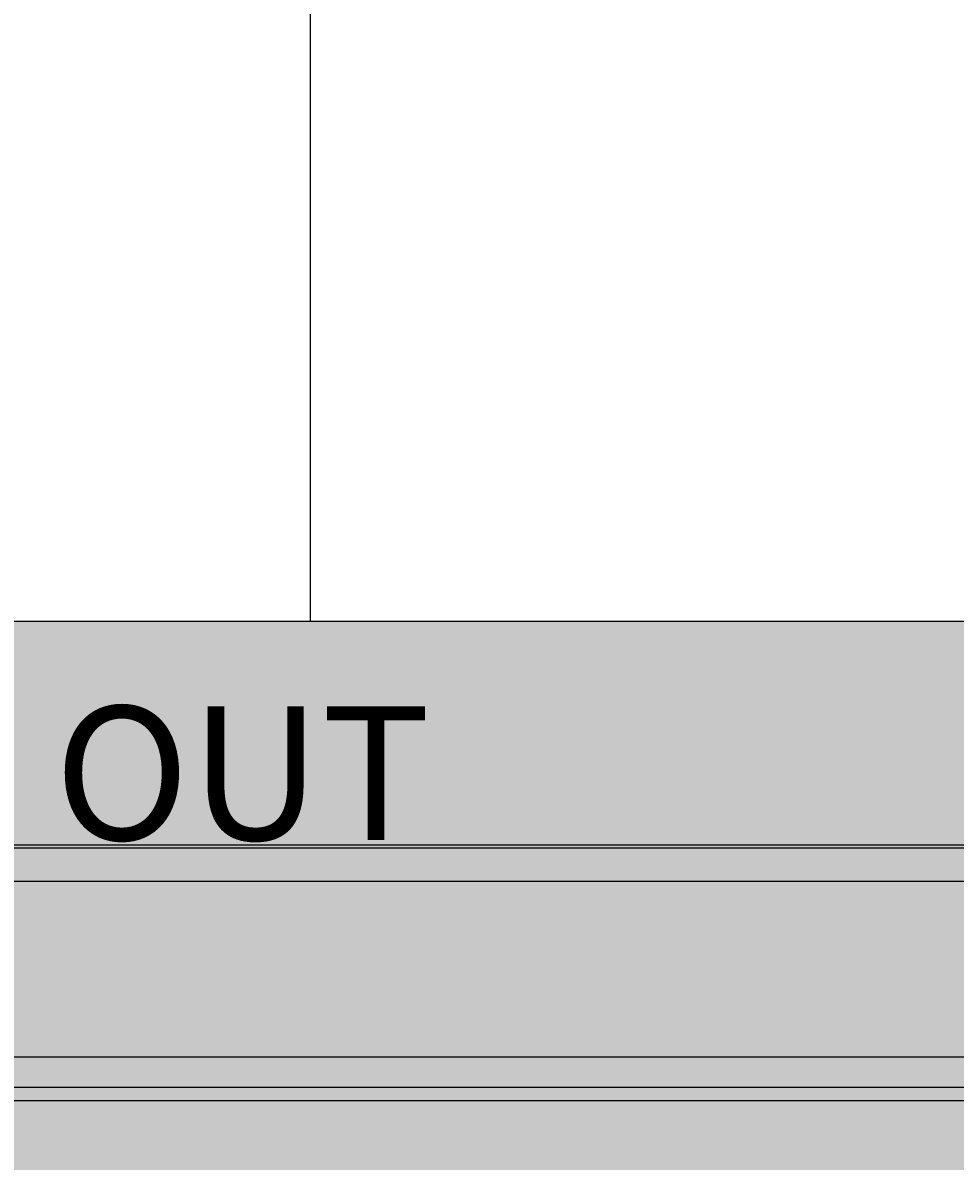
# Model space of a CAD drawing. Units: inches. Extents: x 35362 to 73946, y 43607 to 67532.
# Tile 64 of 134: x 46225 to 47763, y 48798 to 50677. Entities that reach past the tile are written whole.
import ezdxf

# ---------------------------------------------------------------- set-up
doc = ezdxf.new("R2010")
doc.units = ezdxf.units.IN
doc.header["$MEASUREMENT"] = 0
for name, color, linetype, lineweight in [('A-ANNO-DIMS', 2, 'Continuous', 18), ('E-ANNO-TEXT', 5, 'Continuous', 18), ('E-SYMB', 1, 'Continuous', 25), ('E-SYMB-PATT', 1, 'Continuous', 13), ('E-WIRE', 3, 'Continuous', 25)]:
    doc.layers.add(name, color=color, linetype=linetype, lineweight=lineweight)
doc.styles.get("Standard").update_dxf_attribs({"font": 'arial.ttf'})
doc.dimstyles.get("Standard").update_dxf_attribs({"dimtxt": 0.18, "dimasz": 0.18, "dimexe": 0.18, "dimexo": 0.0625, "dimgap": 0.09, "dimtad": 0, "dimtih": 1, "dimtoh": 1, "dimdec": 4, "dimzin": 0, "dimdsep": 46, "dimtxsty": 'Standard', "dimcen": 0.09, "dimadec": 0, "dimazin": 0, "dimtfac": 1, "dimtdec": 4, "dimtofl": 0, "dimtmove": 0, "dimatfit": 3, "dimfxl": 1, "dimtolj": 1, "dimtzin": 0, "dimarcsym": 0})

# ---------------------------------------------------------------- blocks, each defined once
blk = doc.blocks.new('*D40')
at = {"layer": 'A-ANNO-DIMS', "color": 0, "lineweight": -2, "transparency": 16777216}
for p, q in [((56873.5, 53351.5), (35361.8, 53351.5)), ((35361.9, 53351.3), (35361.9, 51333.3)), ((35361.9, 49314.8), (35361.9, 51332.9)), ((51806.5, 49314.7), (35361.8, 49314.7))]:
    blk.add_line(p, q, dxfattribs=at)
at = {"layer": 'A-ANNO-DIMS', "color": 0, "transparency": 16777216}
for points in [[(35361.9, 53351.3), (35362, 53351.3), (35361.9, 53351.5)], [(35361.9, 49314.8), (35362, 49314.8), (35361.9, 49314.7)]]:
    blk.add_solid(points, dxfattribs=at)
at = {"layer": 'Defpoints', "color": 0, "transparency": 16777216}
for p in [(35361.9, 53351.5), (56873.6, 53351.5), (51806.5, 49314.7)]:
    blk.add_point(p, dxfattribs=at)
at = {"layer": 'A-ANNO-DIMS', "color": 0, "transparency": 16777216, "insert": (35361.9, 51333.1), "char_height": 0.18, "attachment_point": 5}
blk.add_mtext('\\A1;4036.9', dxfattribs=at)
blk = doc.blocks.new('*D67')
at = {"layer": 'A-ANNO-DIMS', "color": 0, "lineweight": -2, "transparency": 16777216}
for p, q in [((56873.5, 53351.5), (35361.8, 53351.5)), ((35361.9, 53351.3), (35361.9, 49400.9)), ((35361.9, 45450.1), (35361.9, 49400.5)), ((53793.6, 45449.9), (35361.8, 45449.9))]:
    blk.add_line(p, q, dxfattribs=at)
at = {"layer": 'A-ANNO-DIMS', "color": 0, "transparency": 16777216}
for points in [[(35361.9, 53351.3), (35362, 53351.3), (35361.9, 53351.5)], [(35361.9, 45450.1), (35362, 45450.1), (35361.9, 45449.9)]]:
    blk.add_solid(points, dxfattribs=at)
at = {"layer": 'Defpoints', "color": 0, "transparency": 16777216}
for p in [(35361.9, 53351.5), (56873.6, 53351.5), (53793.6, 45449.9)]:
    blk.add_point(p, dxfattribs=at)
at = {"layer": 'A-ANNO-DIMS', "color": 0, "transparency": 16777216, "insert": (35361.9, 49400.7), "char_height": 0.18, "attachment_point": 5}
blk.add_mtext('\\A1;7901.6', dxfattribs=at)
blk = doc.blocks.new('*D84')
at = {"layer": 'A-ANNO-DIMS', "color": 0, "lineweight": -2, "transparency": 16777216}
for p, q in [((55540.2, 49259.9), (35361.8, 49259.9)), ((35361.9, 49259.8), (35361.9, 49115.1)), ((35361.9, 48970.2), (35361.9, 49114.8)), ((55540.2, 48970), (35361.8, 48970))]:
    blk.add_line(p, q, dxfattribs=at)
at = {"layer": 'A-ANNO-DIMS', "color": 0, "transparency": 16777216}
for points in [[(35361.9, 49259.8), (35362, 49259.8), (35361.9, 49259.9)], [(35361.9, 48970.2), (35362, 48970.2), (35361.9, 48970)]]:
    blk.add_solid(points, dxfattribs=at)
at = {"layer": 'Defpoints', "color": 0, "transparency": 16777216}
for p in [(35361.9, 49259.9), (55540.3, 49259.9), (55540.3, 48970)]:
    blk.add_point(p, dxfattribs=at)
at = {"layer": 'A-ANNO-DIMS', "color": 0, "transparency": 16777216, "insert": (35361.9, 49115), "char_height": 0.18, "attachment_point": 5}
blk.add_mtext('\\A1;289.96', dxfattribs=at)
blk = doc.blocks.new('*D86')
at = {"layer": 'A-ANNO-DIMS', "color": 0, "lineweight": -2, "transparency": 16777216}
for p, q in [((51285.5, 49320.1), (35361.8, 49320.1)), ((35361.9, 49319.9), (35361.9, 49120.3)), ((35361.9, 48920.3), (35361.9, 49119.9)), ((51285.5, 48920.1), (35361.8, 48920.1))]:
    blk.add_line(p, q, dxfattribs=at)
at = {"layer": 'A-ANNO-DIMS', "color": 0, "transparency": 16777216}
for points in [[(35361.9, 49319.9), (35362, 49319.9), (35361.9, 49320.1)], [(35361.9, 48920.3), (35362, 48920.3), (35361.9, 48920.1)]]:
    blk.add_solid(points, dxfattribs=at)
at = {"layer": 'Defpoints', "color": 0, "transparency": 16777216}
for p in [(35361.9, 49320.1), (51285.6, 49320.1), (51285.6, 48920.1)]:
    blk.add_point(p, dxfattribs=at)
at = {"layer": 'A-ANNO-DIMS', "color": 0, "transparency": 16777216, "insert": (35361.9, 49120.1), "char_height": 0.18, "attachment_point": 5}
blk.add_mtext('\\A1;400.0', dxfattribs=at)
blk = doc.blocks.new('*D89')
at = {"layer": 'A-ANNO-DIMS', "color": 0, "lineweight": -2, "transparency": 16777216}
for p, q in [((53707.7, 48897.7), (35361.8, 48897.7)), ((35361.9, 48897.6), (35361.9, 48303.2)), ((35361.9, 47708.4), (35361.9, 48302.8)), ((53707.7, 47708.2), (35361.8, 47708.2))]:
    blk.add_line(p, q, dxfattribs=at)
at = {"layer": 'A-ANNO-DIMS', "color": 0, "transparency": 16777216}
for points in [[(35361.9, 48897.6), (35362, 48897.6), (35361.9, 48897.7)], [(35361.9, 47708.4), (35362, 47708.4), (35361.9, 47708.2)]]:
    blk.add_solid(points, dxfattribs=at)
at = {"layer": 'Defpoints', "color": 0, "transparency": 16777216}
for p in [(53707.8, 48897.7), (35361.9, 47708.2), (53707.8, 47708.2)]:
    blk.add_point(p, dxfattribs=at)
at = {"layer": 'A-ANNO-DIMS', "color": 0, "transparency": 16777216, "insert": (35361.9, 48303), "char_height": 0.18, "attachment_point": 5}
blk.add_mtext('\\A1;1189.5', dxfattribs=at)

msp = doc.modelspace()

# ---------------------------------------------------------------- hatches: boundary and pattern name
at = {"layer": 'E-SYMB-PATT'}
h = msp.add_hatch(color=256, dxfattribs=at)
h.dxf.hatch_style = 1
h.paths.add_polyline_path([(48163.038, 49689.843), (45390.147, 49689.843), (45390.147, 46919.381), (48163.038, 46919.381)])

# ---------------------------------------------------------------- linework, layer by layer
at = {"layer": 'E-SYMB'}
msp.add_lwpolyline([(45390.147, 49689.843), (48163.038, 49689.843), (48163.038, 46919.381), (45390.147, 46919.381)], close=True, dxfattribs=at)
at = {"layer": 'E-WIRE'}
msp.add_line((46698.777, 51529.852), (46698.777, 49689.843), dxfattribs=at)

# ---------------------------------------------------------------- texts
at = {"layer": 'E-ANNO-TEXT'}
msp.add_text('OUT', height=220.866, dxfattribs=at).set_placement((46276.458, 49328.385))

# ---------------------------------------------------------------- dimensions: what is measured, and where the dimension line sits
at = {"layer": 'A-ANNO-DIMS'}
for base, p1, p2, override, picture, middle in [((35361.949, 53351.529), (51806.517, 49314.669), (56873.602, 53351.529), {"dimdec": 1, "dimlfac": 1, "dimrnd": 0, "dimzin": 0, "dimdsep": 46, "dimlunit": 2}, '*D40', (35361.949, 51333.099)), ((35361.949, 53351.529), (53793.638, 45449.894), (56873.602, 53351.529), {"dimdec": 1, "dimlfac": 1, "dimrnd": 0, "dimzin": 0, "dimdsep": 46, "dimlunit": 2}, '*D67', (35361.949, 49400.712)), ((35361.949, 49320.079), (51285.595, 48920.079), (51285.595, 49320.079), {"dimdec": 1, "dimlfac": 1, "dimrnd": 0, "dimzin": 0, "dimdsep": 46, "dimlunit": 2}, '*D86', (35361.949, 49120.079)), ((35361.9491, 49259.9353), (55540.2972, 48969.9796), (55540.2972, 49259.9353), {"dimdec": 2, "dimlfac": 1, "dimrnd": 0, "dimzin": 0, "dimdsep": 46, "dimlunit": 2}, '*D84', (35361.9491, 49114.9575)), ((35361.949, 47708.216), (53707.781, 48897.738), (53707.781, 47708.216), {"dimdec": 1, "dimlfac": 1, "dimrnd": 0, "dimzin": 0, "dimdsep": 46, "dimlunit": 2}, '*D89', (35361.949, 48302.977))]:
    dim = msp.add_linear_dim(base=base, p1=p1, p2=p2, angle=90, dimstyle='Standard', override=override, dxfattribs=at)
    dim.commit()
    dim.dimension.update_dxf_attribs({"geometry": picture, "text_midpoint": middle})

doc.saveas('drawing.dxf')
